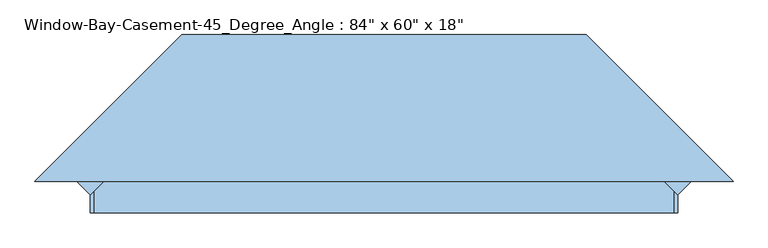
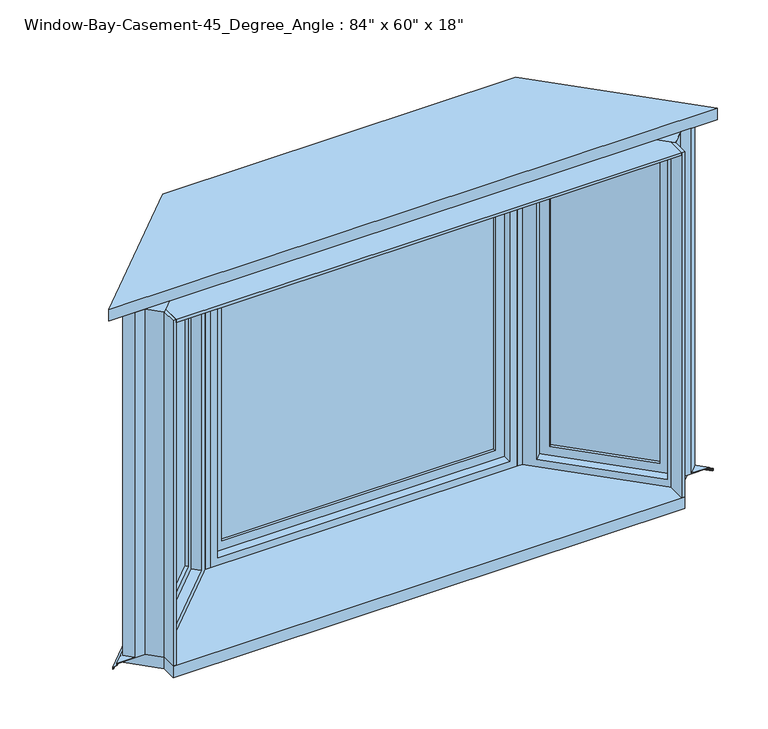
"""IFC4 building model written with IfcOpenShell, lengths in millimetres: window geometry."""

from ifc_helpers import new_model, si_unit, frame, origin, place, context, project, spatial, polyline, outline, extrude, faceted_brep, source, transform, mapped, element, save


def window_f0ba1490(model_context):
    return source(origin(), model_context, "Body", "SolidModel", [
        extrude(outline(polyline([(1066.8, 106.5414087), (1062.3098719, 102.0512806), (771.5637138, 392.7974388), (776.0538418, 397.2875668), (1066.8, 106.5414087)])), frame((0.0, 0.0, 730.25), z_axis=(0.0, 0.0, 1.0), x_axis=(1.0, 0.0, 0.0)), (0.0, 0.0, 1.0), 1384.3),
        extrude(outline(polyline([(1057.8197439, 97.5611525), (1053.3296158, 93.0710245), (762.5834576, 383.8171827), (767.0735857, 388.3073107), (1057.8197439, 97.5611525)])), frame((0.0, 0.0, 730.25), z_axis=(0.0, 0.0, 1.0), x_axis=(1.0, 0.0, 0.0)), (0.0, 0.0, 1.0), 1384.3),
        extrude(outline(polyline([(1441.45, 57.15), (1441.45, -468.3271601), (-57.15, -468.3271601), (-57.15, 57.15), (1441.45, 57.15)]), holes=[polyline([(1384.3, -411.1771601), (1384.3, 0.0), (0.0, 0.0), (0.0, -411.1771601), (1384.3, -411.1771601)])]), frame((1044.3493597, 84.0907684, 730.25), z_axis=(0.7071067811865468, 0.7071067811865483, 0.0), x_axis=(0.0, 0.0, 1.0)), (0.0, 0.0, 1.0), 44.45),
        faceted_brep([(661.8085913, 412.75, 2184.4), (1066.8, 7.7585913, 2184.4), (1116.1914087, 57.15, 2184.4), (1161.0926893, 57.15, 2184.4), (703.8926893, 514.35, 2184.4), (1084.7605122, 43.6796158, 2171.7), (713.192049, 415.2480791, 2171.7), (758.0933296, 460.1493597, 2171.7), (1129.6617928, 88.5808964, 2171.7), (1044.3493597, 30.2092316, 2152.65), (699.7216648, 374.8369265, 2152.65), (726.6624332, 401.7776949, 2152.65), (1071.2901281, 57.15, 2152.65), (713.192049, 415.2480791, 673.1), (758.0933296, 460.1493597, 673.1), (699.7216648, 374.8369265, 692.15), (726.6624332, 401.7776949, 692.15), (703.8926893, 514.35, 660.4), (1161.0926893, 57.15, 660.4), (1116.1914087, 57.15, 660.4), (1066.8, 7.7585913, 660.4), (661.8085913, 412.75, 660.4), (1084.7605122, 43.6796158, 673.1), (1129.6617928, 88.5808964, 673.1), (1044.3493597, 30.2092316, 692.15), (1071.2901281, 57.15, 692.15)], [[[0, 1, 2, 3, 4]], [[5, 6, 7, 8]], [[9, 10, 11, 12]], [[6, 13, 14, 7]], [[10, 15, 16, 11]], [[17, 18, 19, 20, 21]], [[13, 22, 23, 14]], [[15, 24, 25, 16]], [[20, 19, 2, 1]], [[3, 18, 17, 4], [7, 14, 23, 8]], [[8, 23, 22, 5]], [[5, 22, 13, 6], [11, 16, 25, 12]], [[12, 25, 24, 9]], [[1, 0, 21, 20], [9, 24, 15, 10]], [[4, 17, 21, 0]], [[2, 19, 18, 3]]]),
        extrude(outline(polyline([(-1066.8, 106.5414087), (-776.0538418, 397.2875668), (-771.5637138, 392.7974388), (-1062.3098719, 102.0512806), (-1066.8, 106.5414087)])), frame((0.0, 0.0, 730.25), z_axis=(0.0, 0.0, 1.0), x_axis=(1.0, 0.0, 0.0)), (0.0, 0.0, 1.0), 1384.3),
        extrude(outline(polyline([(-1057.8197439, 97.5611525), (-767.0735857, 388.3073107), (-762.5834576, 383.8171827), (-1053.3296158, 93.0710245), (-1057.8197439, 97.5611525)])), frame((0.0, 0.0, 730.25), z_axis=(0.0, 0.0, 1.0), x_axis=(1.0, 0.0, 0.0)), (0.0, 0.0, 1.0), 1384.3),
        extrude(outline(polyline([(1441.45, -57.15), (-57.15, -57.15), (-57.15, 468.3271601), (1441.45, 468.3271601), (1441.45, -57.15)]), holes=[polyline([(1384.3, 411.1771601), (0.0, 411.1771601), (0.0, 0.0), (1384.3, 0.0), (1384.3, 411.1771601)])]), frame((-1044.3493597, 84.0907684, 730.25), z_axis=(-0.7071067811865468, 0.7071067811865483, 0.0), x_axis=(0.0, 0.0, 1.0)), (0.0, 0.0, 1.0), 44.45),
        faceted_brep([(-661.8085913, 412.75, 2184.4), (-703.8926893, 514.35, 2184.4), (-1161.0926893, 57.15, 2184.4), (-1116.1914087, 57.15, 2184.4), (-1066.8, 7.7585913, 2184.4), (-1084.7605122, 43.6796158, 2171.7), (-1129.6617928, 88.5808964, 2171.7), (-758.0933296, 460.1493597, 2171.7), (-713.192049, 415.2480791, 2171.7), (-1044.3493597, 30.2092316, 2152.65), (-1071.2901281, 57.15, 2152.65), (-726.6624332, 401.7776949, 2152.65), (-699.7216648, 374.8369265, 2152.65), (-758.0933296, 460.1493597, 673.1), (-713.192049, 415.2480791, 673.1), (-726.6624332, 401.7776949, 692.15), (-699.7216648, 374.8369265, 692.15), (-703.8926893, 514.35, 660.4), (-661.8085913, 412.75, 660.4), (-1066.8, 7.7585913, 660.4), (-1116.1914087, 57.15, 660.4), (-1161.0926893, 57.15, 660.4), (-1129.6617928, 88.5808964, 673.1), (-1084.7605122, 43.6796158, 673.1), (-1071.2901281, 57.15, 692.15), (-1044.3493597, 30.2092316, 692.15)], [[[0, 1, 2, 3, 4]], [[5, 6, 7, 8]], [[9, 10, 11, 12]], [[8, 7, 13, 14]], [[12, 11, 15, 16]], [[17, 18, 19, 20, 21]], [[14, 13, 22, 23]], [[16, 15, 24, 25]], [[19, 4, 3, 20]], [[2, 1, 17, 21], [7, 6, 22, 13]], [[6, 5, 23, 22]], [[5, 8, 14, 23], [11, 10, 24, 15]], [[10, 9, 25, 24]], [[4, 19, 18, 0], [9, 12, 16, 25]], [[1, 0, 18, 17]], [[3, 2, 21, 20]]]),
        faceted_brep([(-724.9347382, 565.15, 660.4), (-724.9347382, 565.15, 653.0697935), (724.9347382, 565.15, 653.0697935), (724.9347382, 565.15, 660.4), (-703.8926893, 514.35, 663.1486341), (-703.8926893, 514.35, 660.4), (703.8926893, 514.35, 660.4), (703.8926893, 514.35, 663.1486341), (-725.5133946, 566.547, 654.4483503), (-725.5133946, 566.547, 663.1486341), (725.5133946, 566.547, 663.1486341), (725.5133946, 566.547, 654.4483503), (730.7739068, 579.247, 652.2089977), (-730.7739068, 579.247, 652.2089977), (730.7739068, 579.247, 643.2668038), (-730.7739068, 579.247, 643.2668038), (-729.132627, 575.2846, 644.7270038), (-729.132627, 575.2846, 643.2668038), (729.132627, 575.2846, 643.2668038), (729.132627, 575.2846, 644.7270038), (-730.1110823, 577.6468, 650.8662705), (-730.1110823, 577.6468, 644.7270038), (730.1110823, 577.6468, 644.7270038), (730.1110823, 577.6468, 650.8662705), (-1232.9347382, 57.15, 660.4), (-1232.9347382, 57.15, 653.0697935), (1232.9347382, 57.15, 660.4), (1161.0926893, 57.15, 660.4), (-1161.0926893, 57.15, 660.4), (-1161.0926893, 57.15, 663.1486341), (1161.0926893, 57.15, 663.1486341), (1234.9103945, 57.15, 663.1486341), (-1234.9103945, 57.15, 663.1486341), (-1234.9103945, 57.15, 654.4483503), (-1252.8709068, 57.15, 652.2089977), (-1252.8709068, 57.15, 643.2668038), (1252.8709068, 57.15, 643.2668038), (1247.2672271, 57.15, 643.2668038), (-1247.2672271, 57.15, 643.2668038), (-1247.2672271, 57.15, 644.7270038), (1247.2672271, 57.15, 644.7270038), (1250.6078823, 57.15, 644.7270038), (-1250.6078823, 57.15, 644.7270038), (-1250.6078823, 57.15, 650.8662705), (1232.9347382, 57.15, 653.0697935), (1234.9103945, 57.15, 654.4483503), (1252.8709068, 57.15, 652.2089977), (1250.6078823, 57.15, 650.8662705)], [[[0, 1, 2, 3]], [[4, 5, 6, 7]], [[8, 9, 10, 11]], [[8, 11, 12, 13]], [[13, 12, 14, 15]], [[16, 17, 18, 19]], [[20, 21, 22, 23]], [[2, 1, 20, 23]], [[1, 0, 24, 25]], [[0, 3, 26, 27, 6, 5, 28, 24]], [[5, 4, 29, 28]], [[4, 7, 30, 31, 10, 9, 32, 29]], [[9, 8, 33, 32]], [[8, 13, 34, 33]], [[13, 15, 35, 34]], [[15, 14, 36, 37, 18, 17, 38, 35]], [[17, 16, 39, 38]], [[16, 19, 40, 41, 22, 21, 42, 39]], [[21, 20, 43, 42]], [[20, 1, 25, 43]], [[3, 2, 44, 26]], [[7, 6, 27, 30]], [[11, 10, 31, 45]], [[12, 11, 45, 46]], [[14, 12, 46, 36]], [[19, 18, 37, 40]], [[23, 22, 41, 47]], [[2, 23, 47, 44]], [[25, 24, 28, 29, 32, 33, 34, 35, 38, 39, 42, 43]], [[27, 26, 44, 47, 41, 40, 37, 36, 46, 45, 31, 30]]]),
        extrude(outline(polyline([(-1138.642049, 79.6006403), (-1161.0926893, 57.15), (-1192.5235857, 88.5808964), (-1170.0729454, 111.0315367), (-1138.642049, 79.6006403)])), frame((0.0, 0.0, 663.1486341), z_axis=(0.0, 0.0, 1.0), x_axis=(1.0, 0.0, 0.0)), (0.0, 0.0, 1.0), 1521.2513659),
        extrude(outline(polyline([(1138.642049, 79.6006403), (1170.0729454, 111.0315367), (1192.5235857, 88.5808964), (1161.0926893, 57.15), (1138.642049, 79.6006403)])), frame((0.0, 0.0, 663.1486341), z_axis=(0.0, 0.0, 1.0), x_axis=(1.0, 0.0, 0.0)), (0.0, 0.0, 1.0), 1521.2513659),
        extrude(outline(polyline([(735.4557627, 590.55), (1268.8557627, 57.15), (-1268.8557627, 57.15), (-735.4557627, 590.55), (735.4557627, 590.55)])), frame((0.0, 0.0, 2184.4), z_axis=(0.0, 0.0, 1.0), x_axis=(1.0, 0.0, 0.0)), (0.0, 0.0, 1.0), 50.8),
        extrude(outline(polyline([(-639.9414087, 514.35), (-639.9414087, 412.75), (-661.8085913, 412.75), (-703.8926893, 514.35), (-639.9414087, 514.35)])), frame((0.0, 0.0, 660.4), z_axis=(0.0, 0.0, 1.0), x_axis=(1.0, 0.0, 0.0)), (0.0, 0.0, 1.0), 1524.0),
        extrude(outline(polyline([(703.8926893, 514.35), (661.8085913, 412.75), (639.9414087, 412.75), (639.9414087, 514.35), (703.8926893, 514.35)])), frame((0.0, 0.0, 660.4), z_axis=(0.0, 0.0, 1.0), x_axis=(1.0, 0.0, 0.0)), (0.0, 0.0, 1.0), 1524.0),
        faceted_brep([(627.2414087, 450.85, 673.1), (627.2414087, 514.35, 673.1), (-627.2414087, 514.35, 673.1), (-627.2414087, 450.85, 673.1), (608.1914087, 412.75, 692.15), (608.1914087, 450.85, 692.15), (-608.1914087, 450.85, 692.15), (-608.1914087, 412.75, 692.15), (639.9414087, 514.35, 660.4), (639.9414087, 412.75, 660.4), (-639.9414087, 412.75, 660.4), (-639.9414087, 514.35, 660.4), (-627.2414087, 514.35, 2171.7), (-627.2414087, 450.85, 2171.7), (-608.1914087, 450.85, 2152.65), (-608.1914087, 412.75, 2152.65), (-639.9414087, 412.75, 2184.4), (-639.9414087, 514.35, 2184.4), (627.2414087, 514.35, 2171.7), (627.2414087, 450.85, 2171.7), (608.1914087, 450.85, 2152.65), (608.1914087, 412.75, 2152.65), (639.9414087, 412.75, 2184.4), (639.9414087, 514.35, 2184.4)], [[[0, 1, 2, 3]], [[4, 5, 6, 7]], [[8, 9, 10, 11]], [[3, 2, 12, 13]], [[7, 6, 14, 15]], [[11, 10, 16, 17]], [[13, 12, 18, 19]], [[15, 14, 20, 21]], [[17, 16, 22, 23]], [[11, 17, 23, 8], [1, 18, 12, 2]], [[19, 18, 1, 0]], [[3, 13, 19, 0], [5, 20, 14, 6]], [[21, 20, 5, 4]], [[9, 22, 16, 10], [7, 15, 21, 4]], [[23, 22, 9, 8]]]),
        extrude(outline(polyline([(570.0914087, 482.6), (570.0914087, 476.25), (-570.0914087, 476.25), (-570.0914087, 482.6), (570.0914087, 482.6)])), frame((0.0, 0.0, 730.25), z_axis=(0.0, 0.0, 1.0), x_axis=(1.0, 0.0, 0.0)), (0.0, 0.0, 1.0), 1384.3),
        extrude(outline(polyline([(570.0914087, 469.9), (570.0914087, 463.55), (-570.0914087, 463.55), (-570.0914087, 469.9), (570.0914087, 469.9)])), frame((0.0, 0.0, 730.25), z_axis=(0.0, 0.0, 1.0), x_axis=(1.0, 0.0, 0.0)), (0.0, 0.0, 1.0), 1384.3),
        extrude(outline(polyline([(1066.8, -57.15), (-1066.8, -57.15), (-1066.8, 7.7585913), (-1174.5630735, 115.5216648), (-724.9347382, 565.15), (724.9347382, 565.15), (1174.5630735, 115.5216648), (1066.8, 7.7585913), (1066.8, -57.15)])), frame((0.0, 0.0, 609.6), z_axis=(0.0, 0.0, 1.0), x_axis=(1.0, 0.0, 0.0)), (0.0, 0.0, 1.0), 50.8),
        extrude(outline(polyline([(2171.7, -627.2414087), (673.1, -627.2414087), (673.1, 627.2414087), (2171.7, 627.2414087), (2171.7, -627.2414087)]), holes=[polyline([(2114.55, 570.0914087), (730.25, 570.0914087), (730.25, -570.0914087), (2114.55, -570.0914087), (2114.55, 570.0914087)])]), frame((0.0, 450.85, 0.0), z_axis=(0.0, 1.0, 0.0), x_axis=(0.0, 0.0, 1.0)), (0.0, 0.0, 1.0), 44.45),
        extrude(outline(polyline([(-1066.8, -57.15), (-1066.8, 7.7585913), (-1054.1, 20.4585913), (-1054.1, -57.15), (-1066.8, -57.15)])), frame((0.0, 0.0, 660.4), z_axis=(0.0, 0.0, 1.0), x_axis=(1.0, 0.0, 0.0)), (0.0, 0.0, 1.0), 1524.0),
        extrude(outline(polyline([(1066.8, -57.15), (1054.1, -57.15), (1054.1, 20.4585913), (1066.8, 7.7585913), (1066.8, -57.15)])), frame((0.0, 0.0, 660.4), z_axis=(0.0, 0.0, 1.0), x_axis=(1.0, 0.0, 0.0)), (0.0, 0.0, 1.0), 1524.0),
        extrude(outline(polyline([(-661.8085913, 412.75), (661.8085913, 412.75), (1054.1, 20.4585913), (1054.1, -57.15), (-1054.1, -57.15), (-1054.1, 20.4585913), (-661.8085913, 412.75)])), frame((0.0, 0.0, 2171.7), z_axis=(0.0, 0.0, 1.0), x_axis=(1.0, 0.0, 0.0)), (0.0, 0.0, 1.0), 12.7),
    ])


if __name__ == "__main__":
    model = new_model("IFC4")
    model_context = context("Model", 3, world=origin())
    ifc_project = project(units=[si_unit("LENGTHUNIT", "METRE", prefix="MILLI")], contexts=[model_context])
    site = spatial("IfcSite", under=ifc_project)
    building = spatial("IfcBuilding", under=site)
    placement = place(None, origin())
    window_shape = window_f0ba1490(model_context)
    element("IfcWindow", 1, ObjectType="Window-Bay-Casement-45_Degree_Angle : 84\" x 60\" x 18\"", at=placement, inside=building, context=model_context, shape_type="MappedRepresentation", body=[
        mapped(window_shape, transform((0.0, 0.0, 0.0), x_axis=(1.0, 0.0, 0.0), y_axis=(0.0, 1.0, 0.0), z_axis=(0.0, 0.0, 1.0))),
    ])
    save(model, "model.ifc")

# Revit data of these elements
# Type "Window-Bay-Casement-45_Degree_Angle : 84\" x 60\" x 18\""
#   Type Mark = "50"
#   Fire Rating = "0.5h"
#   Assembly Code = "B2020100"
#   Analytic Construction = "Double glazing - domestic"
#   Width of Middle Sash = 4' - 2.38909"
#   Width = 7' - 0"
#   Visual Light Transmittance = 0.81
#   Thermal Resistance (R) = 0.319569 (m²·K)/W
#   Solar Heat Gain Coefficient = 0.76
#   Rough Width = 7' - 0 1/2"
#   Rough Height = 5' - 0 1/2"
#   Length 4 = 0' - 1.13909"
#   Length 3 = 0' - 0.51777"
#   Length 2 = 4' - 7.42462"
#   Length 1 = 1' - 2.80546"
#   Wall Thickness [instance default] = 0' - 6"
#   Trim Width = 7' - 5.03553"
#   Trim Height = 5' - 0"
#   Height 1 = 5' - 2"
#   Height = 5' - 0"
#   Heat Transfer Coefficient (U) = 3.12929 W/(m²·K)
#   Depth = 1' - 6"
#   Default Sill Height = 2' - 0"
#   Angle 1 = 22.50°
#   Angle = 45.00°
#   Center Muntin Visibility = yes
#   Side Muntin Visibility = yes
#   Interior Trim Visibility [instance default] = yes
#   Exterior Trim Visibility [instance default] = yes
#   Center Muntin Pattern = Muntin Pattern_2x2 : Muntin Pattern_2x2
#   Side Muntin Pattern = Muntin Pattern_2x2 : Muntin Pattern_2x2
#   Interior Trim Material = Wood - Stained
#   Exterior Trim Material = Clad - White
#   Exterior Trim = element 339135
#   Interior Trim = Trim-Window-Interior-Flat : Picture Frame
#   Interior Frame Material = Wood - Stained
#   Glass Panel Material = Glass
#   Exterior Frame Material = Clad - White
#   Wall Closure = (empty or 0)
# Element 1 (IfcWindow, "Window-Bay-Casement-45_Degree_Angle : 84\" x 60\" x 18\"")
#   Wall Thickness = 0' - 4 1/2"
#   Materials on its faces: "Wood - Stained", "Clad - White", "Glass"
# Materials
#   "Wood - Stained": class "Wood", colour RGB 227 170 128, transparency 0, Cost = 0
#   "Clad - White": class "Wood", colour RGB 242 242 238, transparency 0, Cost = 0
#   "Glass": class "Glass", colour RGB 0 128 192, transparency 0.9, Description = "Soda Lime Glass", Cost = 0
